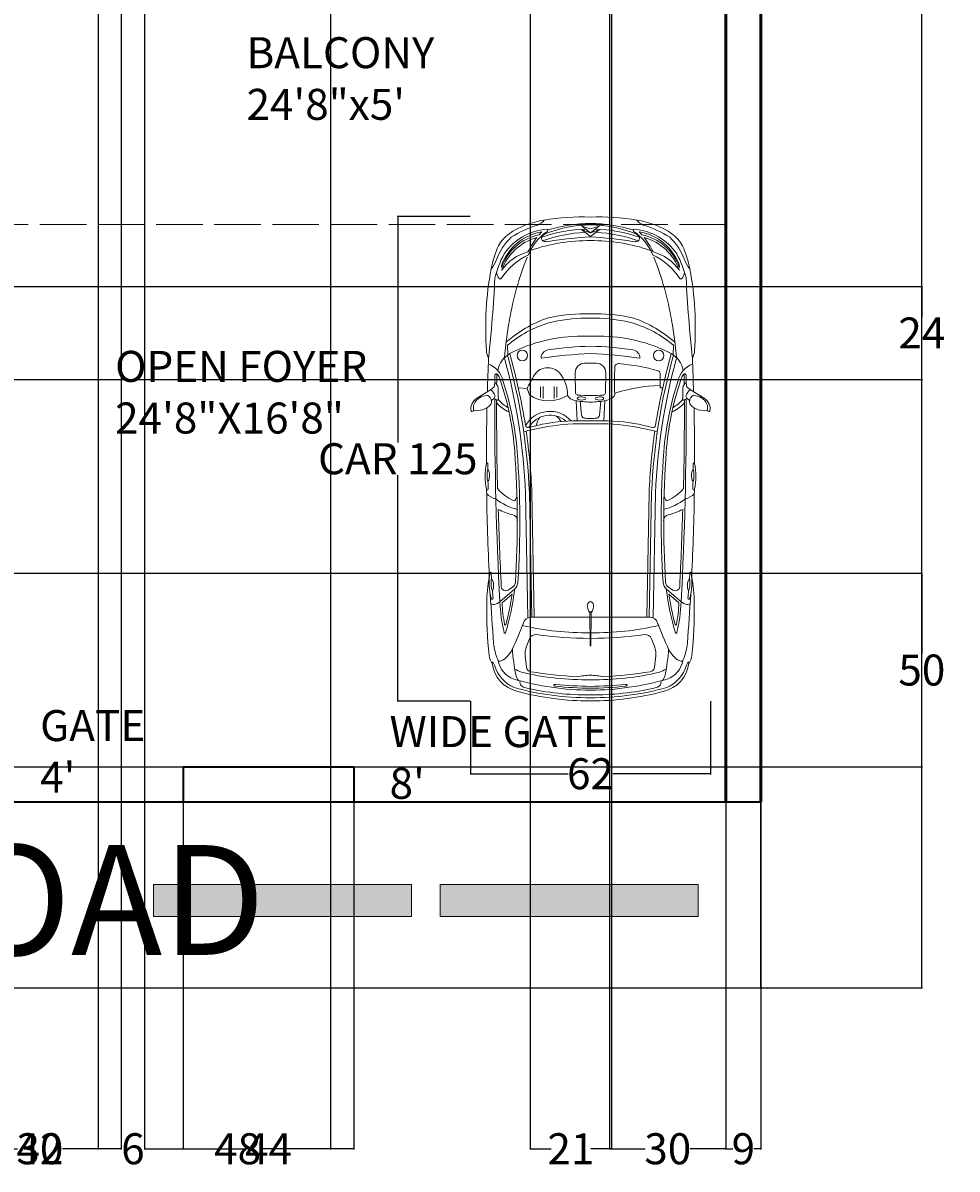
# Model space of a CAD drawing. Units: inches. Extents: x 3004 to 3478, y -798 to 114.
# Tile 2 of 5: x 3232 to 3473, y -798 to -503. Entities that reach past the tile are written whole.
import ezdxf

# ---------------------------------------------------------------- set-up
doc = ezdxf.new("R2010")
doc.units = ezdxf.units.IN
doc.header["$MEASUREMENT"] = 0
doc.linetypes.add('ACAD_ISO02W100', pattern=[15, 12, -3])
for name, color, linetype, lineweight in [('A-ANNO-DIMS', 2, 'Continuous', 18), ('A-ANNO-TEXT', 7, 'Continuous', 18), ('A-AREA-IDEN', 7, 'Continuous', 18), ('A-EQPM-VEHI', 8, 'Continuous', 13), ('A-FLOR-OVHD', 8, 'ACAD_ISO02W100', 18), ('A-WALL', 7, 'Continuous', 50), ('A-WALL-SITE', 7, 'Continuous', 35), ('C-ROAD', 8, 'Continuous', 25), ('C-ROAD-MARK', 8, 'Continuous', 18), ('C-ROAD-PATT', 8, 'Continuous', 13)]:
    doc.layers.add(name, color=color, linetype=linetype, lineweight=lineweight)
doc.styles.get("Standard").update_dxf_attribs({"font": 'arial.ttf', "height": 8})
doc.dimstyles.get("Standard").update_dxf_attribs({"dimtxt": 0.18, "dimasz": 0.18, "dimexe": 0.18, "dimexo": 0.0625, "dimgap": 0.09, "dimtad": 0, "dimtih": 1, "dimtoh": 1, "dimzin": 0, "dimdsep": 46, "dimlunit": 4, "dimtxsty": 'Standard', "dimcen": 0.09, "dimadec": 0, "dimazin": 0, "dimtfac": 1, "dimtofl": 0, "dimtmove": 0, "dimatfit": 3, "dimfxl": 1, "dimtolj": 1, "dimtzin": 0, "dimarcsym": 0})

# ---------------------------------------------------------------- blocks, each defined once
blk = doc.blocks.new('A$C2B1738E4')
for p, q in [((1.3752, 1.7441), (1.4407, 1.8548)), ((1.4589, 1.7386), (1.441, 1.7168)), ((0.3886, 1.659), (0.4009, 1.6583)), ((2.9607, 1.5544), (3.0621, 1.6708)), ((2.9998, 1.5734), (3.0696, 1.6535)), ((1.021, 1.6102), (1.0959, 1.6067)), ((2.9449, 1.5699), (2.9683, 1.606)), ((1.3603, 1.5062), (1.3588, 1.5242)), ((1.708, 1.4786), (1.6826, 1.3685)), ((2.1966, 1.4663), (3.1889, 1.4476)), ((3.3555, 1.4354), (3.4233, 1.4605)), ((3.5828, 1.459), (3.4918, 1.469)), ((1.6741, 1.4428), (1.6582, 1.3741)), ((2.1955, 1.4163), (3.1845, 1.3977)), ((2.1961, 1.4363), (3.1849, 1.4177)), ((3.1849, 0.955), (3.1849, 1.4259)), ((0.1249, 0.95), (0.0716, 1.0196)), ((0.0949, 0.95), (0.0716, 1.0196)), ((0.155, 0.95), (0.1016, 1.0196)), ((0.1249, 0.95), (0.1016, 1.0196)), ((0.9477, 0.95), (0.9477, 1.0156)), ((1.2395, 1.0714), (1.4016, 1.069)), ((1.4617, 1.0641), (1.6212, 1.0565)), ((1.4665, 1.0328), (1.5781, 1.0213)), ((1.6211, 0.95), (1.6211, 1.0484)), ((1.6461, 0.95), (1.6461, 1.0484)), ((0.1249, 0.95), (0.0716, 0.8804)), ((0.0949, 0.95), (0.0716, 0.8804)), ((0.155, 0.95), (0.1016, 0.8804)), ((0.1249, 0.95), (0.1016, 0.8804)), ((0.7701, 0.9987), (0.7701, 0.95)), ((0.7701, 0.9013), (0.7701, 0.95)), ((0.8055, 0.9872), (0.8055, 0.95)), ((0.8055, 0.9128), (0.8055, 0.95)), ((0.9477, 0.95), (0.9477, 0.8844)), ((1.1634, 0.95), (1.1634, 0.9965)), ((1.1634, 0.95), (1.1634, 0.9035)), ((1.6211, 0.95), (1.6211, 0.8516)), ((1.6461, 0.95), (1.6461, 0.8516)), ((3.1468, 0.9554), (3.41, 0.953)), ((3.1468, 0.9446), (3.41, 0.947)), ((3.1849, 0.9449), (3.1849, 0.4741)), ((1.2395, 0.8286), (1.4016, 0.831)), ((1.4617, 0.8359), (1.6212, 0.8435)), ((1.4665, 0.8672), (1.5781, 0.8787)), ((1.3479, 0.6598), (1.4429, 0.6598)), ((1.3504, 0.6818), (1.4354, 0.6818)), ((1.3479, 0.5738), (1.4429, 0.5738)), ((1.3504, 0.5518), (1.4354, 0.5518)), ((1.4152, 0.4645), (1.3649, 0.4464)), ((1.6741, 0.4572), (1.6582, 0.5259)), ((1.708, 0.4213), (1.6826, 0.5315)), ((2.1955, 0.4837), (3.1845, 0.5023)), ((2.1961, 0.4637), (3.1849, 0.4823)), ((3.3555, 0.4646), (3.4233, 0.4395)), ((1.3649, 0.4464), (1.3588, 0.3758)), ((2.1966, 0.4337), (3.1889, 0.4524)), ((3.5828, 0.441), (3.4918, 0.431)), ((1.021, 0.2898), (1.0959, 0.2933)), ((2.9449, 0.3301), (2.9683, 0.294)), ((2.9607, 0.3456), (3.0621, 0.2292)), ((2.9998, 0.3266), (3.0696, 0.2465)), ((0.3886, 0.241), (0.4009, 0.2417)), ((1.4589, 0.1614), (1.441, 0.1832)), ((1.3752, 0.1559), (1.4407, 0.0452))]:
    blk.add_line(p, q)
for centre in [(1.1021, 1.4921), (1.1021, 0.4079)]:
    blk.add_circle(centre, 0.042)
for centre, radius, start, end in [((1.5378, 1.7696), 0.1177, 114.90167, 178.70982), ((1.5464, 1.7751), 0.1324, 115.73664, 142.9787), ((1.5174, 1.7983), 0.0834, 74.27488, 110.49282), ((1.5238, 1.8221), 0.0802, 75.99437, 115.81785), ((1.383, 1.8572), 0.1584, 315.10581, 7.73883), ((1.4975, 1.9069), 0.0511, 326.30655, 345.23611), ((1.542, 1.8951), 0.005, 345.23611, 75.99437), ((0.5639, 0.9554), 0.7996, 100.82935, 114.76098), ((0.2753, 1.8979), 0.2094, 287.71329, 311.36331), ((0.8815, -0.7709), 2.5548, 85.91634, 100.5502), ((-0.0763, 13.0836), 11.3867, 272.81583, 276.05051), ((1.0641, 1.6643), 0.1131, 58.06404, 90.32501), ((1.9324, -16.8508), 18.6287, 91.6668, 92.4874), ((1.3435, 1.8252), 0.1838, 200.02457, 256.74778), ((1.4909, 1.6361), 0.1583, 136.95388, 146.46292), ((1.4437, 1.7882), 0.0815, 212.77688, 252.78841), ((1.44, 1.7718), 0.02, 178.70982, 218.46095), ((1.4694, 1.7951), 0.0574, 218.46095, 288.23064), ((1.4811, 1.7595), 0.02, 288.23064, 315.10581), ((1.9324, -16.8508), 18.6287, 89.89266, 91.27658), ((1.9621, 1.7715), 0.005, 103.42644, 270.21117), ((2.0673, 1.3309), 0.458, 77.46788, 103.42644), ((1.9865, -4.8499), 6.6164, 89.84025, 90.21117), ((2.0532, 1.5772), 0.1954, 74.52362, 104.28787), ((2.056, 1.8524), 0.0999, 239.25719, 299.5543), ((1.9865, -4.8499), 6.6164, 88.45454, 88.97124), ((2.1651, 1.7711), 0.007, 268.45454, 77.46788), ((1.9324, -16.8508), 18.6287, 87.14394, 89.26971), ((2.1008, 1.6687), 0.1466, 13.42369, 47.02054), ((2.8314, 1.7457), 0.005, 99.69218, 266.47692), ((2.9076, 1.2992), 0.458, 73.73362, 99.69218), ((2.4245, -4.8632), 6.6164, 86.106, 86.47692), ((3.0784, 0.5679), 1.2067, 90.09348, 100.39783), ((2.9096, 1.5459), 0.1954, 70.78937, 100.55362), ((2.9304, 1.8203), 0.0999, 235.52294, 295.82004), ((1.9324, -16.8508), 18.6287, 85.51048, 86.70458), ((3.034, 1.7321), 0.007, 264.72029, 73.73362), ((3.1484, -1.132), 2.9075, 83.29074, 91.41866), ((3.05, 1.7232), 0.0339, 341.73176, 34.91983), ((3.4758, 1.6117), 0.1444, 56.27191, 85.11868), ((0.5243, 1.2709), 0.4112, 109.27565, 170.59544), ((0.3723, 1.4211), 0.2972, 118.82253, 143.4182), ((0.5375, 1.2777), 0.4043, 109.74736, 168.44654), ((0.5034, 1.2578), 0.4703, 110.45328, 136.60155), ((0.5625, 1.2664), 0.4141, 109.497, 164.5583), ((0.6414, 1.3497), 0.3761, 125.2539, 164.96052), ((0.7203, 0.8185), 0.9232, 104.89425, 117.56498), ((0.7769, 1.2167), 0.5278, 122.97123, 154.50043), ((0.397, 1.5452), 0.1605, 54.62031, 73.38017), ((0.4842, 1.6679), 0.01, 302.97123, 54.62031), ((1.2618, 1.4887), 0.2036, 101.57607, 149.41971), ((1.2594, 1.6989), 0.012, 90.48413, 236.34536), ((1.3435, 1.8252), 0.1638, 236.34536, 252.50294), ((1.2589, 1.6909), 0.005, 90.48527, 237.79054), ((1.5079, -27.7125), 29.4094, 90.34567, 90.48527), ((1.5079, -27.7125), 29.4244, 90.35553, 90.48413), ((2.0306, 3.8274), 2.2805, 251.1637, 265.95801), ((2.0945, 4.13), 2.6072, 252.29101, 265.02186), ((1.3263, 1.7064), 0.005, 111.52507, 225.42537), ((1.3672, 1.7478), 0.0632, 225.42537, 277.32143), ((1.3431, 1.6638), 0.0508, 90.69796, 111.52507), ((1.3423, 1.7346), 0.02, 270.69796, 326.46292), ((1.3434, 0.0126), 1.6729, 86.48872, 88.90928), ((1.4255, 1.7295), 0.02, 252.78841, 320.66271), ((1.4172, 1.6843), 0.0403, 15.34561, 53.84194), ((1.4464, 1.6923), 0.01, 266.48872, 15.34561), ((1.5079, -27.7125), 29.4244, 86.97218, 90.11938), ((1.2866, 1.4767), 0.2643, 29.12459, 51.49342), ((1.5079, -27.7125), 29.4094, 88.72931, 90.10212), ((1.2866, 1.4767), 0.2913, 24.55248, 49.10987), ((1.9273, 1.412), 0.3623, 24.58813, 50.02619), ((1.8936, 1.4263), 0.4458, 13.66567, 38.31453), ((1.871, 1.4494), 0.5127, 13.35508, 27.16426), ((1.5079, -27.7125), 29.4074, 87.20739, 88.40354), ((2.939, 1.625), 0.035, 327.00754, 87.20739), ((2.4245, -4.8632), 6.6164, 84.72029, 85.23699), ((2.9667, 1.7425), 0.1193, 323.10117, 345.48476), ((3.0163, 0.453), 1.2187, 76.14889, 87.84658), ((3.0163, 0.453), 1.2017, 79.14037, 87.46029), ((3.3395, 1.2332), 0.4902, 68.10598, 84.02503), ((3.3572, 1.7536), 0.1987, 293.56008, 331.9101), ((3.5149, 1.6695), 0.02, 331.9101, 68.10598), ((3.4986, 1.4979), 0.1889, 19.3672, 81.0133), ((3.547, 1.7278), 0.005, 84.11827, 238.27251), ((3.592, 1.8007), 0.0907, 238.27251, 253.64287), ((3.5208, 1.4743), 0.2598, 12.15586, 84.11827), ((3.4944, 1.4544), 0.2691, 22.30479, 74.45895), ((0.6564, 1.2351), 0.6365, 145.21739, 172.37744), ((0.9608, 1.0781), 0.9441, 147.82068, 161.82152), ((0.5546, 1.2586), 0.4598, 124.65571, 174.9915), ((1.2632, -0.9334), 2.567, 99.86714, 111.58903), ((1.7226, 0.9769), 0.9705, 138.40536, 160.95232), ((1.4961, -2.3385), 3.9912, 95.40573, 99.70466), ((1.7346, 1.0079), 0.9337, 139.83465, 162.91734), ((2.2149, 1.0156), 1.2672, 152.92654, 180), ((2.4912, 6.6298), 5.2296, 254.41947, 260.8306), ((2.396, 6.2265), 4.7944, 254.30377, 267.61053), ((2.4043, 6.3103), 4.8485, 254.64174, 267.554), ((2.4266, 9.0701), 7.5381, 265.76426, 273.64732), ((2.2113, 1.5979), 0.0634, 276.39096, 314.37154), ((2.2477, 1.5586), 0.01, 322.45289, 24.58813), ((2.4153, 1.5786), 0.0467, 193.35508, 269.91364), ((2.903, 1.5971), 0.05, 273.64732, 327.00754), ((2.9004, 1.6069), 0.08, 275.05795, 318.93156), ((2.7162, 3.568), 2.0297, 276.88198, 286.96439), ((2.7162, 3.568), 2.0147, 278.09202, 285.1628), ((2.6245, 3.2042), 1.8236, 289.37801, 296.44539), ((3.2418, 1.6283), 0.005, 285.1628, 79.14037), ((3.3069, 1.6314), 0.005, 286.96439, 76.14889), ((3.303, -0.265), 1.8411, 79.39083, 85.84555), ((3.3327, 1.3998), 0.3053, 18.91715, 30.01108), ((1.5376, 0.9391), 2.2276, 0.27964, 16.19876), ((1.6997, 0.9728), 2.1253, 359.38445, 15.94069), ((2.9698, 1.0062), 1.8116, 164.57186, 174.60708), ((1.2428, 1.4829), 0.02, 89.97833, 164.57186), ((1.2677, 67.4361), 65.9332, 269.978328, 270.077881), ((2.7086, 1.5526), 1.3696, 182.07953, 197.42099), ((1.3573, 1.5059), 0.003, 270.07788, 4.93143), ((1.6546, 1.4473), 0.02, 347.00555, 80.8306), ((2.396, 6.2265), 4.8144, 261.73884, 267.61326), ((2.4266, 9.0701), 7.5581, 265.76327, 273.64732), ((3.2449, 1.4259), 0.06, 104.73425, 180), ((1.1524, 0.9926), 2.1558, 358.97289, 13.37296), ((3.4754, 1.3199), 0.15, 83.74198, 110.33677), ((1.5744, 0.9967), 2.1077, 358.73151, 13.7827), ((3.613, 1.427), 0.1212, 52.0949, 76.1783), ((3.7024, 1.4743), 0.0377, 39.75104, 107.96998), ((3.6527, 1.4403), 0.0979, 13.89286, 36.45625), ((1.5466, 0.9695), 2.2559, 359.50384, 12.65584), ((1.7073, 0.9663), 2.1428, 359.56434, 15.22514), ((-0.0346, 1.4031), 0.103, 305.74578, 342.7889), ((0.4477, 1.0741), 0.3981, 111.71191, 146.73951), ((0.5331, 0.9039), 0.6002, 115.13155, 128.02582), ((1.6436, 0.96), 1.4556, 161.24905, 180.39424), ((3.0696, 1.0484), 1.4484, 167.00555, 180), ((3.0696, 1.0484), 1.4234, 167.00555, 180), ((3.3729, 1.3885), 0.05, 110.33677, 187.78064), ((0.1551, 0.9488), 3.1977, 0.0842, 7.78064), ((3.5785, 1.4192), 0.04, 8.86829, 83.74198), ((-0.7599, 0.7423), 4.4308, 4.0656, 8.86829), ((1.7762, 1.0128), 1.7773, 170.0606, 182.02372), ((1.2451, 0.9417), 1.1934, 163.10645, 179.60049), ((1.0709, 0.9361), 1.0084, 158.13259, 179.21161), ((0.1065, 1.2979), 0.01, 174.9915, 326.73951), ((1.2113, 0.9687), 1.1144, 160.6158, 179.09365), ((0.5331, 0.9039), 0.6002, 130.7339, 133.66821), ((1.3263, 0.9274), 1.2066, 160.47738, 176.85471), ((0.2015, 1.28), 0.0737, 132.92762, 154.49597), ((0.1685, 1.3124), 0.0275, 34.40383, 128.49042), ((2.8191, 0.8287), 2.663, 170.19968, 177.38825), ((0.1134, 1.2985), 0.0831, 348.52278, 20.75628), ((2.0282, 0.9987), 1.258, 166.43803, 180), ((2.0149, 0.9872), 1.2094, 165.88293, 180), ((4.4096, 0.8275), 3.3845, 172.21398, 177.92575), ((1.122, 1.2761), 0.0664, 87.82641, 171.40523), ((4.4696, 0.8275), 3.3845, 171.24819, 177.92575), ((3.7302, 1.2308), 0.0117, 120.01215, 187.552), ((0.6607, 0.9129), 3.0742, 0.69091, 5.90586), ((3.7256, 1.2347), 0.00632, 29.97799, 102.2567), ((3.7057, 1.226), 0.0281, 6.55416, 24.97983), ((0.6757, 0.9129), 3.0742, 0.69091, 5.90586), ((1.1961, 1.1737), 0.03, 174.60708, 266.77269), ((1.3098, 3.1905), 2.05, 266.77269, 272.70056), ((1.4078, 1.1128), 0.03, 40.48904, 92.70056), ((1.3272, 1.044), 0.136, 12.59064, 40.48904), ((1.2384, 0.9965), 0.075, 89.13616, 180), ((1.4013, 1.054), 0.015, 3.83938, 89.13616), ((-1.0819, 0.8874), 2.5039, 1.43373, 3.83938), ((0.7063, 0.9317), 0.7669, 1.36752, 10.66295), ((1.5755, 0.9964), 0.025, 8.91242, 84.13426), ((4.2548, 0.9205), 0.6104, 167.13037, 177.23004), ((1.7762, 0.8872), 1.7773, 177.97628, 189.9394), ((1.2451, 0.9583), 1.1934, 180.39951, 196.89355), ((1.0709, 0.9639), 1.0084, 180.78839, 201.86741), ((1.2113, 0.9313), 1.1144, 180.90635, 199.3842), ((1.3263, 0.9274), 1.2066, 178.26552, 178.62581), ((1.3263, 0.9726), 1.2066, 181.37419, 181.73448), ((2.8191, 1.0713), 2.663, 182.61175, 189.80032), ((1.6436, 0.94), 1.4556, 179.60576, 198.75095), ((2.0149, 0.9128), 1.2094, 180, 194.11707), ((4.4096, 1.0725), 3.3845, 182.07425, 187.78602), ((4.4696, 1.0725), 3.3845, 182.07425, 188.75181), ((-1.0819, 1.0126), 2.5039, 356.16062, 358.56627), ((0.7063, 0.9683), 0.7669, 349.33705, 358.63248), ((1.2433, 0.9443), 0.3613, 0.89844, 8.91242), ((1.2433, 0.9557), 0.3613, 351.08758, 359.10156), ((3.0907, 0.9414), 0.0324, 99.63608, 164.53559), ((3.0907, 0.9586), 0.0324, 195.46441, 260.36392), ((3.0957, 0.8943), 0.0797, 50.07633, 97.53265), ((3.0957, 1.0057), 0.0797, 262.46735, 309.92367), ((3.1468, 0.95), 0.0054, 88.95657, 271.04343), ((1.1524, 0.9074), 2.1558, 346.62704, 1.02711), ((0.1551, 0.9512), 3.1977, 352.21936, 359.9158), ((3.41, 0.95), 0.003, 359.99996, 89.47828), ((3.41, 0.95), 0.003, 270.52172, 0.00004), ((1.5744, 0.9033), 2.1077, 346.2173, 1.26849), ((4.2548, 0.9795), 0.6104, 182.76996, 192.86963), ((1.5376, 0.9609), 2.2276, 343.80124, 359.72036), ((0.6607, 0.9871), 3.0742, 354.09414, 359.30909), ((0.6757, 0.9871), 3.0742, 354.09414, 359.30909), ((1.6997, 0.9272), 2.1253, 344.05931, 0.61555), ((1.5466, 0.9305), 2.2559, 347.34416, 0.49616), ((1.7073, 0.9337), 2.1428, 344.77486, 0.43566), ((1.3263, 0.9726), 1.2066, 183.14529, 199.52262), ((2.0282, 0.9013), 1.258, 180, 193.56197), ((2.2149, 0.8844), 1.2672, 180, 207.07346), ((1.2384, 0.9035), 0.075, 180, 270.86384), ((1.4013, 0.846), 0.015, 270.86384, 356.16062), ((1.3735, 0.8412), 0.0877, 301.69002, 350.31009), ((1.5755, 0.9036), 0.025, 275.86574, 351.08758), ((3.0696, 0.8516), 1.4484, 180, 192.99445), ((3.0696, 0.8516), 1.4234, 180, 192.99445), ((-0.7599, 1.1577), 4.4308, 351.13171, 355.9344), ((1.4118, 0.5019), 0.2647, 88.32025, 129.77769), ((1.1939, 0.6187), 0.2698, 325.11832, 33.22242), ((1.7692, 0.6276), 0.2228, 131.27466, 240.64488), ((1.7692, 0.6276), 0.1928, 138.70172, 240.1859), ((1.3264, 0.6101), 0.1269, 131.39571, 242.86676), ((1.6923, 0.5951), 0.1361, 118.39383, 143.81944), ((3.7302, 0.6692), 0.0117, 172.448, 239.98785), ((3.7256, 0.6653), 0.00632, 257.7433, 330.02201), ((3.7057, 0.674), 0.0281, 335.02017, 353.44584), ((0.6564, 0.6649), 0.6365, 187.62256, 214.78261), ((-0.0346, 0.4969), 0.103, 17.2111, 54.25422), ((0.1065, 0.6021), 0.01, 33.26049, 185.0085), ((0.5546, 0.6414), 0.4598, 185.0085, 235.34429), ((0.4477, 0.8259), 0.3981, 213.26049, 248.28809), ((0.5331, 0.9961), 0.6002, 226.33179, 229.2661), ((0.5243, 0.6291), 0.4112, 189.40456, 250.72435), ((0.2015, 0.62), 0.0737, 205.50403, 227.07238), ((0.1685, 0.5876), 0.0275, 231.50958, 325.59617), ((0.1134, 0.6015), 0.0831, 339.24372, 11.47722), ((1.7226, 0.9231), 0.9705, 199.04768, 221.59464), ((1.7346, 0.8921), 0.9337, 197.08266, 220.16535), ((1.122, 0.6239), 0.0664, 188.59477, 272.17359), ((1.6786, 0.6519), 0.1341, 230.62849, 261.94999), ((0.9608, 0.8219), 0.9441, 198.17848, 212.17932), ((0.5375, 0.6223), 0.4043, 191.55346, 250.25264), ((0.5625, 0.6336), 0.4141, 195.4417, 250.503), ((0.5331, 0.9961), 0.6002, 231.97418, 244.86845), ((0.7769, 0.6833), 0.5278, 205.49957, 237.02877), ((2.396, -4.3265), 4.7944, 92.38947, 105.69623), ((1.7409, 1.2774), 0.9121, 238.8071, 245.65365), ((1.6546, 0.4527), 0.02, 279.1694, 12.99445), ((2.396, -4.3265), 4.8144, 92.38674, 98.26116), ((3.2449, 0.4741), 0.06, 180, 255.26575), ((3.3729, 0.5115), 0.05, 172.21936, 249.66323), ((3.5785, 0.4808), 0.04, 276.25802, 351.13171), ((0.6414, 0.5503), 0.3761, 195.03948, 234.7461), ((1.2632, 2.8334), 2.567, 248.41097, 260.13286), ((2.4912, -4.7298), 5.2296, 99.1694, 105.58053), ((2.4043, -4.4103), 4.8485, 92.446, 105.35826), ((2.0945, -2.23), 2.6072, 94.97814, 107.70899), ((2.4266, -7.1701), 7.5581, 86.35268, 94.23673), ((2.4266, -7.1701), 7.5381, 86.35268, 94.23574), ((2.2113, 0.3021), 0.0634, 45.62846, 83.60904), ((1.8936, 0.4737), 0.4458, 321.68547, 346.33433), ((2.4153, 0.3214), 0.0467, 90.08636, 166.64492), ((2.9004, 0.2931), 0.08, 41.06844, 84.94205), ((2.6245, -1.3042), 1.8236, 63.55461, 70.62199), ((3.4754, 0.5801), 0.15, 249.66323, 276.25802), ((3.5208, 0.4257), 0.2598, 275.88173, 347.84414), ((3.3327, 0.5002), 0.3053, 329.98892, 341.08285), ((3.613, 0.473), 0.1212, 283.8217, 307.9051), ((3.7024, 0.4257), 0.0377, 252.03002, 320.24896), ((3.6527, 0.4597), 0.0979, 323.54375, 346.10714), ((0.3723, 0.4789), 0.2972, 216.5818, 241.17747), ((0.5034, 0.6422), 0.4703, 223.39845, 249.54672), ((1.4961, 4.2385), 3.9912, 260.29534, 264.59427), ((1.2618, 0.4113), 0.2036, 210.58029, 258.42393), ((2.0306, -1.9274), 2.2805, 94.04199, 108.8363), ((1.2866, 0.4233), 0.2643, 308.50658, 330.87541), ((1.2866, 0.4233), 0.2913, 310.89013, 335.44752), ((1.9273, 0.488), 0.3623, 309.97381, 335.41187), ((2.2477, 0.3414), 0.01, 335.41187, 37.54711), ((1.871, 0.4506), 0.5127, 332.83574, 346.64492), ((2.903, 0.3029), 0.05, 32.99246, 86.35268), ((2.939, 0.275), 0.035, 272.79261, 32.99246), ((2.7162, -1.668), 2.0297, 73.03561, 83.11802), ((2.7162, -1.668), 2.0147, 74.8372, 81.90798), ((3.2418, 0.2717), 0.005, 280.85963, 74.8372), ((3.303, 2.165), 1.8411, 274.15445, 280.60917), ((3.3572, 0.1464), 0.1987, 28.0899, 66.43992), ((3.4986, 0.4021), 0.1889, 278.9867, 340.6328), ((3.4944, 0.4456), 0.2691, 285.54105, 337.69521), ((0.5639, 0.9446), 0.7996, 245.23902, 259.17065), ((0.7203, 1.0815), 0.9232, 242.43502, 255.10575), ((0.2753, 0.0021), 0.2094, 48.63669, 72.28671), ((0.397, 0.3548), 0.1605, 286.61983, 305.37969), ((-0.0763, -11.1836), 11.3867, 83.94949, 87.18417), ((0.4842, 0.2321), 0.01, 305.37969, 57.02877), ((1.3435, 0.0748), 0.1838, 103.25222, 159.97543), ((1.2594, 0.2011), 0.012, 123.65464, 269.51587), ((1.3435, 0.0748), 0.1638, 107.49706, 123.65464), ((1.2589, 0.2091), 0.005, 122.20946, 269.51473), ((1.5079, 29.6125), 29.4094, 269.51473, 269.65433), ((1.5079, 29.6125), 29.4244, 269.51587, 269.64447), ((1.3263, 0.1936), 0.005, 134.57463, 248.47493), ((1.3672, 0.1522), 0.0632, 82.67857, 134.57463), ((1.3431, 0.2362), 0.0508, 248.47493, 269.30204), ((1.3423, 0.1654), 0.02, 33.53708, 89.30204), ((1.3434, 1.8874), 1.6729, 271.09072, 273.51128), ((1.4437, 0.1118), 0.0815, 107.21159, 147.22312), ((1.4255, 0.1705), 0.02, 39.33729, 107.21159), ((1.4172, 0.2157), 0.0403, 306.15806, 344.65439), ((1.4464, 0.2077), 0.01, 344.65439, 93.51128), ((1.5079, 29.6125), 29.4244, 269.88062, 273.02782), ((1.5079, 29.6125), 29.4094, 269.89788, 271.27069), ((2.1008, 0.2313), 0.1466, 312.97946, 346.57631), ((1.5079, 29.6125), 29.4074, 271.59646, 272.79261), ((3.0163, 1.447), 1.2187, 272.15342, 283.85111), ((2.9667, 0.1575), 0.1193, 14.51524, 36.89883), ((3.0163, 1.447), 1.2017, 272.53971, 280.85963), ((3.05, 0.1768), 0.0339, 325.08017, 18.26824), ((3.3069, 0.2686), 0.005, 283.85111, 73.03561), ((3.3395, 0.6668), 0.4902, 275.97497, 291.89402), ((3.5149, 0.2305), 0.02, 291.89402, 28.0899), ((3.592, 0.0993), 0.0907, 106.35713, 121.72749), ((0.8815, 2.6709), 2.5548, 259.4498, 274.08366), ((1.0641, 0.2357), 0.1131, 269.67499, 301.93596), ((1.9324, 18.7508), 18.6287, 267.5126, 268.3332), ((1.4909, 0.2639), 0.1583, 213.53708, 223.04612), ((1.44, 0.1282), 0.02, 141.53905, 181.29018), ((1.5378, 0.1304), 0.1177, 181.29018, 245.09833), ((1.4694, 0.1049), 0.0574, 71.76936, 141.53905), ((1.4811, 0.1405), 0.02, 44.89419, 71.76936), ((1.383, 0.0428), 0.1584, 352.26117, 44.89419), ((1.9324, 18.7508), 18.6287, 268.72342, 270.10734), ((1.9621, 0.1285), 0.005, 89.78883, 256.57356), ((2.0673, 0.5691), 0.458, 256.57356, 282.53212), ((1.9865, 6.7499), 6.6164, 269.78883, 270.15975), ((2.056, 0.0476), 0.0999, 60.4457, 120.74281), ((2.0532, 0.3228), 0.1954, 255.71213, 285.47638), ((1.9865, 6.7499), 6.6164, 271.02876, 271.54546), ((2.1651, 0.1289), 0.007, 282.53212, 91.54546), ((1.9324, 18.7508), 18.6287, 270.73029, 272.85606), ((2.8314, 0.1543), 0.005, 93.52308, 260.30782), ((2.9076, 0.6008), 0.458, 260.30782, 286.26638), ((2.4245, 6.7632), 6.6164, 273.52308, 273.894), ((3.0784, 1.3321), 1.2067, 259.60217, 269.90652), ((2.9304, 0.0797), 0.0999, 64.17996, 124.47706), ((2.9096, 0.3541), 0.1954, 259.44638, 289.21063), ((2.4245, 6.7632), 6.6164, 274.76301, 275.27971), ((1.9324, 18.7508), 18.6287, 273.29542, 274.48952), ((3.034, 0.1679), 0.007, 286.26638, 95.27971), ((3.1484, 3.032), 2.9075, 268.58134, 276.70926), ((3.4758, 0.2883), 0.1444, 274.88132, 303.72809), ((3.547, 0.1722), 0.005, 121.72749, 275.88173), ((1.5464, 0.1249), 0.1324, 217.0213, 244.26336), ((1.5174, 0.1017), 0.0834, 249.50718, 285.72512), ((1.5238, 0.0779), 0.0802, 244.18215, 284.00563), ((1.4975, -0.0069), 0.0511, 14.76389, 33.69345), ((1.542, 0.0049), 0.005, 284.00563, 14.76389)]:
    blk.add_arc(centre, radius, start, end)
at = {"extrusion": (0, 0, -1)}
blk.add_ellipse((1.4437, 1.0222), major_axis=(-0.0013, 0.0351), ratio=0.355056, dxfattribs=at)
blk.add_ellipse((1.4437, 0.8778), major_axis=(-0.0013, -0.0351), ratio=0.355056)
blk = doc.blocks.new('*D28')
at = {"layer": 'A-ANNO-DIMS', "color": 0, "lineweight": -2, "transparency": 16777216}
for p, q in [((3347.25, -552.61), (3328.37, -552.61)), ((3328.55, -552.79), (3328.55, -610.92)), ((3328.55, -677.5), (3328.55, -619.37)), ((3347.25, -677.68), (3328.37, -677.68))]:
    blk.add_line(p, q, dxfattribs=at)
at = {"layer": 'A-ANNO-DIMS', "color": 0, "transparency": 16777216}
for points in [[(3328.52, -552.79), (3328.58, -552.79), (3328.55, -552.61)], [(3328.52, -677.5), (3328.58, -677.5), (3328.55, -677.68)]]:
    blk.add_solid(points, dxfattribs=at)
at = {"layer": 'Defpoints', "color": 0, "transparency": 16777216}
for p in [(3347.31, -552.61), (3328.55, -677.68), (3347.31, -677.68)]:
    blk.add_point(p, dxfattribs=at)
at = {"layer": 'A-ANNO-DIMS', "color": 0, "transparency": 16777216, "insert": (3328.55, -615.14), "char_height": 8, "attachment_point": 5}
blk.add_mtext('\\A1;CAR 125', dxfattribs=at)
blk = doc.blocks.new('*D29')
at = {"layer": 'A-ANNO-DIMS', "color": 0, "lineweight": -2, "transparency": 16777216}
for p, q in [((3347.31, -677.74), (3347.31, -696.62)), ((3409.23, -677.74), (3409.23, -696.62)), ((3347.49, -696.44), (3372.47, -696.44)), ((3409.05, -696.44), (3384.07, -696.44))]:
    blk.add_line(p, q, dxfattribs=at)
at = {"layer": 'A-ANNO-DIMS', "color": 0, "transparency": 16777216}
for points in [[(3347.49, -696.41), (3347.49, -696.47), (3347.31, -696.44)], [(3409.05, -696.41), (3409.05, -696.47), (3409.23, -696.44)]]:
    blk.add_solid(points, dxfattribs=at)
at = {"layer": 'Defpoints', "color": 0, "transparency": 16777216}
for p in [(3347.31, -677.68), (3409.23, -677.68), (3409.23, -696.44)]:
    blk.add_point(p, dxfattribs=at)
at = {"layer": 'A-ANNO-DIMS', "color": 0, "transparency": 16777216, "insert": (3378.27, -696.44), "char_height": 8, "attachment_point": 5}
blk.add_mtext('\\A1;62', dxfattribs=at)
blk = doc.blocks.new('*D39')
at = {"layer": 'A-ANNO-DIMS', "color": 0, "lineweight": -2, "transparency": 16777216}
for p, q in [((3422.27, 16.32), (3463.94, 16.32)), ((3463.76, 16.14), (3463.76, -363.5)), ((3463.76, -751.5), (3463.76, -371.85)), ((3422.27, -751.68), (3463.94, -751.68))]:
    blk.add_line(p, q, dxfattribs=at)
at = {"layer": 'A-ANNO-DIMS', "color": 0, "transparency": 16777216}
for points in [[(3463.73, 16.14), (3463.79, 16.14), (3463.76, 16.32)], [(3463.73, -751.5), (3463.79, -751.5), (3463.76, -751.68)]]:
    blk.add_solid(points, dxfattribs=at)
at = {"layer": 'Defpoints', "color": 0, "transparency": 16777216}
for p in [(3422.21, 16.32), (3422.21, -751.68), (3463.76, -751.68)]:
    blk.add_point(p, dxfattribs=at)
at = {"layer": 'A-ANNO-DIMS', "color": 0, "transparency": 16777216, "insert": (3463.76, -367.68), "char_height": 8, "attachment_point": 5}
blk.add_mtext('\\A1;768', dxfattribs=at)
blk = doc.blocks.new('*D43')
at = {"layer": 'A-ANNO-DIMS', "color": 0, "lineweight": -2, "transparency": 16777216}
for p, q in [((3273.21, -694.74), (3273.21, -793.41)), ((3317.21, -694.74), (3317.21, -793.41)), ((3273.39, -793.23), (3289.25, -793.23)), ((3317.03, -793.23), (3301.18, -793.23))]:
    blk.add_line(p, q, dxfattribs=at)
at = {"layer": 'A-ANNO-DIMS', "color": 0, "transparency": 16777216}
for points in [[(3273.39, -793.2), (3273.39, -793.26), (3273.21, -793.23)], [(3317.03, -793.2), (3317.03, -793.26), (3317.21, -793.23)]]:
    blk.add_solid(points, dxfattribs=at)
at = {"layer": 'Defpoints', "color": 0, "transparency": 16777216}
for p in [(3273.21, -694.68), (3317.21, -694.68), (3317.21, -793.23)]:
    blk.add_point(p, dxfattribs=at)
at = {"layer": 'A-ANNO-DIMS', "color": 0, "transparency": 16777216, "insert": (3295.21, -793.23), "char_height": 8, "attachment_point": 5}
blk.add_mtext('\\A1;44', dxfattribs=at)
blk = doc.blocks.new('*D44')
at = {"layer": 'A-ANNO-DIMS', "color": 0, "lineweight": -2, "transparency": 16777216}
for p, q in [((3257.211316, -220.74039), (3257.211316, -793.40789)), ((3263.211316, -220.74039), (3263.211316, -793.40789)), ((3257.031316, -793.22789), (3256.851316, -793.22789)), ((3263.391316, -793.22789), (3263.571316, -793.22789))]:
    blk.add_line(p, q, dxfattribs=at)
at = {"layer": 'A-ANNO-DIMS', "color": 0, "transparency": 16777216}
for points in [[(3257.031316, -793.19789), (3257.031316, -793.25789), (3257.211316, -793.22789)], [(3263.391316, -793.19789), (3263.391316, -793.25789), (3263.211316, -793.22789)]]:
    blk.add_solid(points, dxfattribs=at)
at = {"layer": 'Defpoints', "color": 0, "transparency": 16777216}
for p in [(3257.211316, -220.67789), (3263.211316, -220.67789), (3263.211316, -793.22789)]:
    blk.add_point(p, dxfattribs=at)
at = {"layer": 'A-ANNO-DIMS', "color": 0, "transparency": 16777216, "insert": (3260.211316, -793.22789), "char_height": 8, "attachment_point": 5}
blk.add_mtext('\\A1;6', dxfattribs=at)
blk = doc.blocks.new('*D45')
at = {"layer": 'A-ANNO-DIMS', "color": 0, "lineweight": -2, "transparency": 16777216}
for p, q in [((3422.21, 16.26), (3422.21, -793.41)), ((3413.21, 7.26), (3413.21, -793.41)), ((3413.39, -793.23), (3414.99, -793.23)), ((3422.03, -793.23), (3420.43, -793.23))]:
    blk.add_line(p, q, dxfattribs=at)
at = {"layer": 'A-ANNO-DIMS', "color": 0, "transparency": 16777216}
for points in [[(3413.39, -793.2), (3413.39, -793.26), (3413.21, -793.23)], [(3422.03, -793.2), (3422.03, -793.26), (3422.21, -793.23)]]:
    blk.add_solid(points, dxfattribs=at)
at = {"layer": 'Defpoints', "color": 0, "transparency": 16777216}
for p in [(3422.21, 16.32), (3413.21, 7.32), (3422.21, -793.23)]:
    blk.add_point(p, dxfattribs=at)
at = {"layer": 'A-ANNO-DIMS', "color": 0, "transparency": 16777216, "insert": (3417.71, -793.23), "char_height": 8, "attachment_point": 5}
blk.add_mtext('\\A1;9', dxfattribs=at)
blk = doc.blocks.new('*D46')
at = {"layer": 'A-ANNO-DIMS', "color": 0, "lineweight": -2, "transparency": 16777216}
for p, q in [((3263.21, -214.34), (3263.21, -793.41)), ((3311.21, -214.74), (3311.21, -793.41)), ((3263.39, -793.23), (3281.22, -793.23)), ((3311.03, -793.23), (3293.2, -793.23))]:
    blk.add_line(p, q, dxfattribs=at)
at = {"layer": 'A-ANNO-DIMS', "color": 0, "transparency": 16777216}
for points in [[(3263.39, -793.2), (3263.39, -793.26), (3263.21, -793.23)], [(3311.03, -793.2), (3311.03, -793.26), (3311.21, -793.23)]]:
    blk.add_solid(points, dxfattribs=at)
at = {"layer": 'Defpoints', "color": 0, "transparency": 16777216}
for p in [(3263.21, -214.28), (3311.21, -214.68), (3311.21, -793.23)]:
    blk.add_point(p, dxfattribs=at)
at = {"layer": 'A-ANNO-DIMS', "color": 0, "transparency": 16777216, "insert": (3287.21, -793.23), "char_height": 8, "attachment_point": 5}
blk.add_mtext('\\A1;48', dxfattribs=at)
blk = doc.blocks.new('*D47')
at = {"layer": 'A-ANNO-DIMS', "color": 0, "lineweight": -2, "transparency": 16777216}
for p, q in [((3413.21, -42.74), (3413.21, -793.41)), ((3383.21, -46.74), (3383.21, -793.41)), ((3383.39, -793.23), (3392.41, -793.23)), ((3413.03, -793.23), (3404.01, -793.23))]:
    blk.add_line(p, q, dxfattribs=at)
at = {"layer": 'A-ANNO-DIMS', "color": 0, "transparency": 16777216}
for points in [[(3383.39, -793.2), (3383.39, -793.26), (3383.21, -793.23)], [(3413.03, -793.2), (3413.03, -793.26), (3413.21, -793.23)]]:
    blk.add_solid(points, dxfattribs=at)
at = {"layer": 'Defpoints', "color": 0, "transparency": 16777216}
for p in [(3413.21, -42.68), (3383.21, -46.68), (3413.21, -793.23)]:
    blk.add_point(p, dxfattribs=at)
at = {"layer": 'A-ANNO-DIMS', "color": 0, "transparency": 16777216, "insert": (3398.21, -793.23), "char_height": 8, "attachment_point": 5}
blk.add_mtext('\\A1;30', dxfattribs=at)
blk = doc.blocks.new('*D56')
at = {"layer": 'A-ANNO-DIMS', "color": 0, "lineweight": -2, "transparency": 16777216}
for p, q in [((3213.27, -644.68), (3463.94, -644.68)), ((3463.76, -644.86), (3463.76, -665.5)), ((3463.76, -694.5), (3463.76, -673.85)), ((3213.27, -694.68), (3463.94, -694.68))]:
    blk.add_line(p, q, dxfattribs=at)
at = {"layer": 'A-ANNO-DIMS', "color": 0, "transparency": 16777216}
for points in [[(3463.73, -644.86), (3463.79, -644.86), (3463.76, -644.68)], [(3463.73, -694.5), (3463.79, -694.5), (3463.76, -694.68)]]:
    blk.add_solid(points, dxfattribs=at)
at = {"layer": 'Defpoints', "color": 0, "transparency": 16777216}
for p in [(3213.21, -644.68), (3213.21, -694.68), (3463.76, -694.68)]:
    blk.add_point(p, dxfattribs=at)
at = {"layer": 'A-ANNO-DIMS', "color": 0, "transparency": 16777216, "insert": (3463.76, -669.68), "char_height": 8, "attachment_point": 5}
blk.add_mtext('\\A1;50', dxfattribs=at)
blk = doc.blocks.new('*D58')
at = {"layer": 'A-ANNO-DIMS', "color": 0, "lineweight": -2, "transparency": 16777216}
for p, q in [((3117.27, -570.68), (3463.94, -570.68)), ((3463.76, -570.86), (3463.76, -578.57)), ((3463.76, -594.5), (3463.76, -586.78)), ((3117.27, -594.68), (3463.94, -594.68))]:
    blk.add_line(p, q, dxfattribs=at)
at = {"layer": 'A-ANNO-DIMS', "color": 0, "transparency": 16777216}
for points in [[(3463.73, -570.86), (3463.79, -570.86), (3463.76, -570.68)], [(3463.73, -594.5), (3463.79, -594.5), (3463.76, -594.68)]]:
    blk.add_solid(points, dxfattribs=at)
at = {"layer": 'Defpoints', "color": 0, "transparency": 16777216}
for p in [(3117.21, -570.68), (3117.21, -594.68), (3463.76, -594.68)]:
    blk.add_point(p, dxfattribs=at)
at = {"layer": 'A-ANNO-DIMS', "color": 0, "transparency": 16777216, "insert": (3463.76, -582.68), "char_height": 8, "attachment_point": 5}
blk.add_mtext('\\A1;24', dxfattribs=at)
blk = doc.blocks.new('*D59')
at = {"layer": 'A-ANNO-DIMS', "color": 0, "lineweight": -2, "transparency": 16777216}
for p, q in [((3362.72, -0.74), (3362.72, -793.41)), ((3383.72, -0.74), (3383.72, -793.41)), ((3362.9, -793.23), (3368.1, -793.23)), ((3383.54, -793.23), (3378.33, -793.23))]:
    blk.add_line(p, q, dxfattribs=at)
at = {"layer": 'A-ANNO-DIMS', "color": 0, "transparency": 16777216}
for points in [[(3362.9, -793.2), (3362.9, -793.26), (3362.72, -793.23)], [(3383.54, -793.2), (3383.54, -793.26), (3383.72, -793.23)]]:
    blk.add_solid(points, dxfattribs=at)
at = {"layer": 'Defpoints', "color": 0, "transparency": 16777216}
for p in [(3362.72, -0.68), (3383.72, -0.68), (3383.72, -793.23)]:
    blk.add_point(p, dxfattribs=at)
at = {"layer": 'A-ANNO-DIMS', "color": 0, "transparency": 16777216, "insert": (3373.22, -793.23), "char_height": 8, "attachment_point": 5}
blk.add_mtext('\\A1;21', dxfattribs=at)
blk = doc.blocks.new('*D63')
at = {"layer": 'A-ANNO-DIMS', "color": 0, "lineweight": -2, "transparency": 16777216}
for p, q in [((3221.21, -46.74), (3221.21, -793.41)), ((3251.21, -46.74), (3251.21, -793.41)), ((3221.39, -793.23), (3230.41, -793.23)), ((3251.03, -793.23), (3242.01, -793.23))]:
    blk.add_line(p, q, dxfattribs=at)
at = {"layer": 'A-ANNO-DIMS', "color": 0, "transparency": 16777216}
for points in [[(3221.39, -793.2), (3221.39, -793.26), (3221.21, -793.23)], [(3251.03, -793.2), (3251.03, -793.26), (3251.21, -793.23)]]:
    blk.add_solid(points, dxfattribs=at)
at = {"layer": 'Defpoints', "color": 0, "transparency": 16777216}
for p in [(3221.21, -46.68), (3251.21, -46.68), (3251.21, -793.23)]:
    blk.add_point(p, dxfattribs=at)
at = {"layer": 'A-ANNO-DIMS', "color": 0, "transparency": 16777216, "insert": (3236.21, -793.23), "char_height": 8, "attachment_point": 5}
blk.add_mtext('\\A1;30', dxfattribs=at)
blk = doc.blocks.new('*D64')
at = {"layer": 'A-ANNO-DIMS', "color": 0, "lineweight": -2, "transparency": 16777216}
for p, q in [((3215.21, -190.74), (3215.21, -793.41)), ((3257.21, -220.74), (3257.21, -793.41)), ((3215.39, -793.23), (3230.27, -793.23)), ((3257.03, -793.23), (3242.15, -793.23))]:
    blk.add_line(p, q, dxfattribs=at)
at = {"layer": 'A-ANNO-DIMS', "color": 0, "transparency": 16777216}
for points in [[(3215.39, -793.2), (3215.39, -793.26), (3215.21, -793.23)], [(3257.03, -793.2), (3257.03, -793.26), (3257.21, -793.23)]]:
    blk.add_solid(points, dxfattribs=at)
at = {"layer": 'Defpoints', "color": 0, "transparency": 16777216}
for p in [(3215.21, -190.68), (3257.21, -220.68), (3257.21, -793.23)]:
    blk.add_point(p, dxfattribs=at)
at = {"layer": 'A-ANNO-DIMS', "color": 0, "transparency": 16777216, "insert": (3236.21, -793.23), "char_height": 8, "attachment_point": 5}
blk.add_mtext('\\A1;42', dxfattribs=at)

msp = doc.modelspace()

# ---------------------------------------------------------------- hatches: boundary and pattern name
at = {"layer": 'C-ROAD-PATT'}
h = msp.add_hatch(color=256, dxfattribs=at)
h.dxf.hatch_style = 1
h.paths.add_polyline_path([(3134.8245, -725.0263), (3068.2428, -725.0263), (3068.2428, -733.2952), (3134.8245, -733.2952)])
h.paths.add_polyline_path([(3217.7696, -725.0263), (3151.1878, -725.0263), (3151.1878, -733.2952), (3217.7696, -733.2952)])
h.paths.add_polyline_path([(3180.7889, -759.1898), (3309.3973, -759.1898), (3309.3973, -700.7648), (3180.7889, -700.7648)], flags=9)
h = msp.add_hatch(color=256, dxfattribs=at)
h.dxf.hatch_style = 1
h.paths.add_polyline_path([(3406.0421, -725.0263), (3339.4603, -725.0263), (3339.4603, -733.2952), (3406.0421, -733.2952)])
h.paths.add_polyline_path([(3332.0926, -725.0263), (3265.5108, -725.0263), (3265.5108, -733.2952), (3332.0926, -733.2952)])
h.paths.add_polyline_path([(3180.7889, -759.1898), (3309.3973, -759.1898), (3309.3973, -700.7648), (3180.7889, -700.7648)], flags=9)

# ---------------------------------------------------------------- linework, layer by layer
at = {"layer": 'A-FLOR-OVHD'}
msp.add_line((3413.2113, -554.6779), (3113.2113, -554.6779), dxfattribs=at)
at = {"layer": 'A-WALL'}
for p, q in [((3422.2113, 16.3221), (3422.2113, -703.6779)), ((3413.2113, 7.3221), (3413.2113, -703.6779))]:
    msp.add_line(p, q, dxfattribs=at)
at = {"layer": 'A-WALL-SITE'}
for p, q in [((3273.2113, -694.6779), (3273.2113, -703.6779)), ((3273.2113, -694.6779), (3317.2113, -694.6779)), ((3317.2113, -694.6779), (3317.2113, -703.6779)), ((3062.2113, -703.6779), (3422.2113, -703.6779))]:
    msp.add_line(p, q, dxfattribs=at)
at = {"layer": 'C-ROAD'}
for p, q in [((3422.2113, -751.6779), (3422.2113, -703.6779)), ((3062.2113, -751.6779), (3422.2113, -751.6779))]:
    msp.add_line(p, q, dxfattribs=at)
at = {"layer": 'C-ROAD-MARK'}
for points in [[(3265.5108, -725.0263), (3332.0926, -725.0263), (3332.0926, -733.2952), (3265.5108, -733.2952)], [(3339.4603, -725.0263), (3406.0421, -725.0263), (3406.0421, -733.2952), (3339.4603, -733.2952)]]:
    msp.add_lwpolyline(points, close=True, dxfattribs=at)

# ---------------------------------------------------------------- block references
at = {"layer": 'A-EQPM-VEHI', "xscale": 32.43609714528208, "yscale": 32.43609714528208, "zscale": 32.43609714528208, "rotation": 270}
msp.add_blockref('A$C2B1738E4', (3347.4574, -552.7513), dxfattribs=at)

# ---------------------------------------------------------------- texts
at = {"layer": 'A-ANNO-TEXT', "attachment_point": 1}
for s, width, gutter_width, insert, char_height in [("GATE\\P4'", 228.23715, 40, (3236.278, -680.0189), 8), ("WIDE GATE\\P8'", 228.23715, 40, (3326.4321, -681.583), 8), ('ROAD', 577.293337, 141.7594, (3190.9905, -714.8537), 28.35188)]:
    msp.add_mtext_dynamic_manual_height_columns(s, width=width, gutter_width=gutter_width, heights=[0], dxfattribs=dict(at, insert=insert, char_height=char_height))
at = {"layer": 'A-AREA-IDEN', "char_height": 8, "attachment_point": 1}
for s, insert in [('BALCONY\\P24\'8"x5\'', (3289.5179, -506.3425)), ('OPEN FOYER\\P24\'8"X16\'8"', (3255.6238, -587.3027))]:
    msp.add_mtext_dynamic_manual_height_columns(s, width=228.23715, gutter_width=40, heights=[0], dxfattribs=dict(at, insert=insert))

# ---------------------------------------------------------------- dimensions: what is measured, and where the dimension line sits
at = {"layer": 'A-ANNO-DIMS'}
for base, p1, p2, picture, middle in [((3422.2113, -793.2279), (3413.2113, 7.3221), (3422.2113, 16.3221), '*D45', (3417.7113, -793.2279)), ((3383.7177, -793.2279), (3362.7177, -0.6779), (3383.7177, -0.6779), '*D59', (3373.2177, -793.2279)), ((3413.2113, -793.2279), (3383.2113, -46.6779), (3413.2113, -42.6779), '*D47', (3398.2113, -793.2279)), ((3251.2113, -793.2279), (3221.2113, -46.6779), (3251.2113, -46.6779), '*D63', (3236.2113, -793.2279)), ((3257.2113, -793.2279), (3215.2113, -190.6779), (3257.2113, -220.6779), '*D64', (3236.2113, -793.2279)), ((3311.2113, -793.2279), (3263.2113, -214.2779), (3311.2113, -214.6779), '*D46', (3287.2113, -793.2279)), ((3263.2113, -793.2279), (3257.2113, -220.6779), (3263.2113, -220.6779), '*D44', (3260.2113, -793.2279)), ((3409.2329, -696.4387), (3347.3104, -677.6783), (3409.2329, -677.6783), '*D29', (3378.2717, -696.4387)), ((3317.2113, -793.2279), (3273.2113, -694.6779), (3317.2113, -694.6779), '*D43', (3295.2113, -793.2279))]:
    dim = msp.add_linear_dim(base=base, p1=p1, p2=p2, dimstyle='Standard', override={"dimdec": 0, "dimlfac": 1, "dimrnd": 0, "dimzin": 0, "dimdsep": 46, "dimlunit": 2}, dxfattribs=at)
    dim.commit()
    dim.dimension.update_dxf_attribs({"geometry": picture, "text_midpoint": middle})
for base, p1, p2, picture, middle in [((3463.7613, -751.6779), (3422.2113, 16.3221), (3422.2113, -751.6779), '*D39', (3463.7613, -367.6779)), ((3463.7613, -594.6779), (3117.2113, -570.6779), (3117.2113, -594.6779), '*D58', (3463.7613, -582.6779)), ((3463.7613, -694.6779), (3213.2113, -644.6779), (3213.2113, -694.6779), '*D56', (3463.7613, -669.6779))]:
    dim = msp.add_linear_dim(base=base, p1=p1, p2=p2, angle=90, dimstyle='Standard', override={"dimdec": 0, "dimlfac": 1, "dimrnd": 0, "dimzin": 0, "dimdsep": 46, "dimlunit": 2}, dxfattribs=at)
    dim.commit()
    dim.dimension.update_dxf_attribs({"geometry": picture, "text_midpoint": middle})
dim = msp.add_linear_dim(base=(3328.5501, -677.6783), p1=(3347.3104, -552.6093), p2=(3347.3104, -677.6783), angle=270, text='CAR <>', dimstyle='Standard', override={"dimdec": 0, "dimlfac": 1, "dimrnd": 0, "dimzin": 0, "dimdsep": 46, "dimlunit": 2}, dxfattribs=at)
dim.commit()
dim.dimension.update_dxf_attribs({"geometry": '*D28', "text_midpoint": (3328.5501, -615.1438)})

doc.saveas('drawing.dxf')
